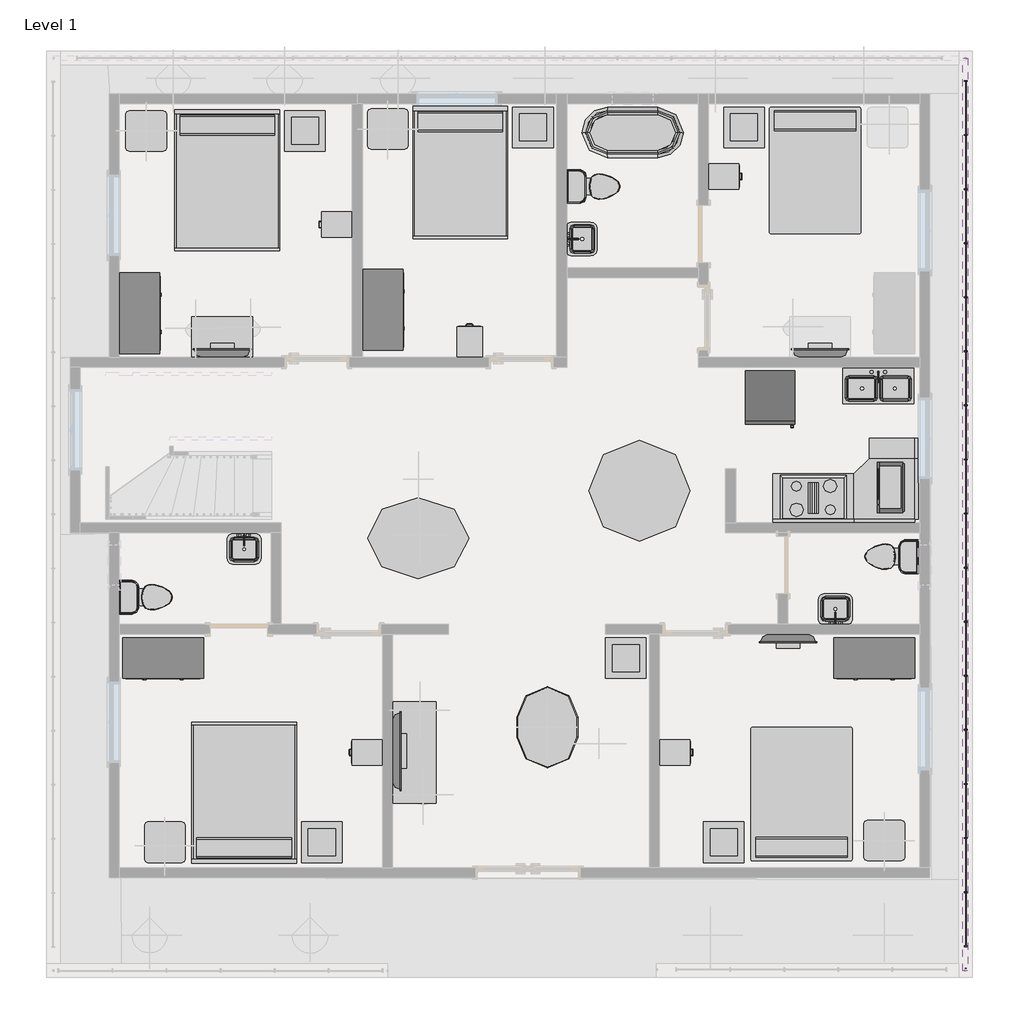
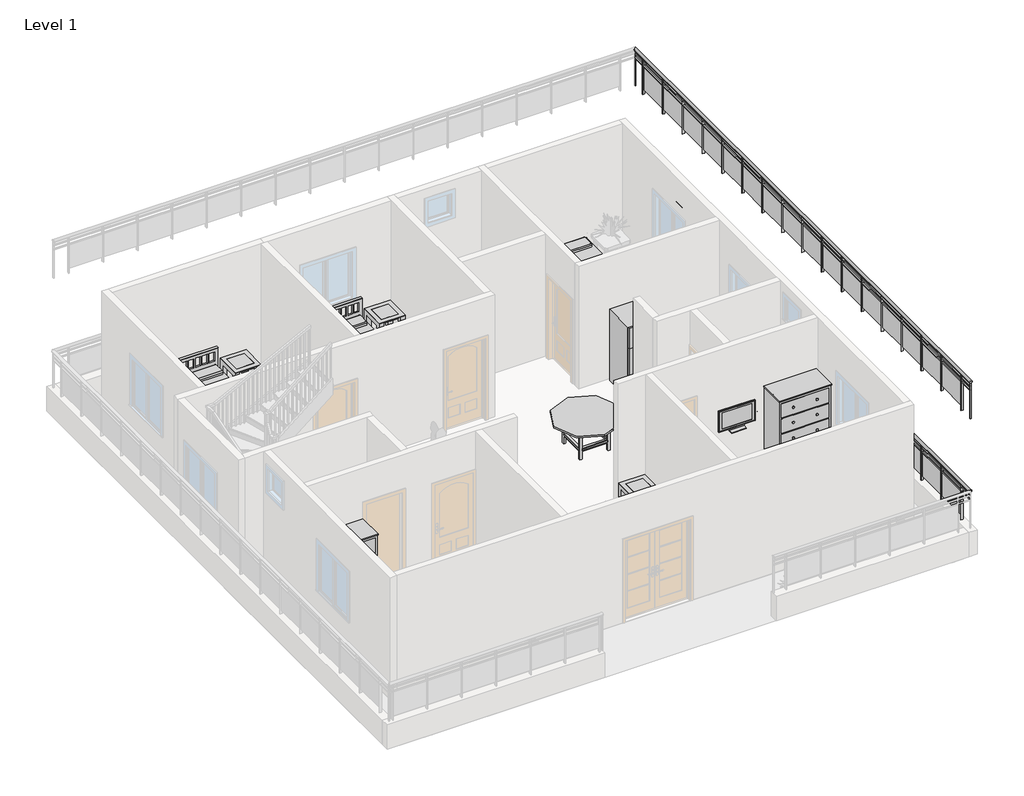
# One storey, part 4 of 5: 34 furniture elements, 11 flow terminals, 3 proxies, 2 railings.
"""IFC4 building model written with IfcOpenShell, lengths in millimetres."""

from ifc_helpers import new_model, si_unit, point, frame, origin, place, context, project, spatial, polyline, ellipse_curve, trimmed, outline, extrude, transform, mapped, element, save
from ifc_brep_helpers import plane_surface, extruded_surface, advanced_brep
from components import proxy_bb1e6e30, proxy_8a8d5ab2, proxy_a13a33b2, flow_terminal_accce45a, flow_terminal_a53be723, flow_terminal_62a433f7, toilet_domestic_3d_toilet_domestic_3d_f7549cf7, toilet_domestic_3d_toilet_domestic_3d_183bbd19, flow_terminal_b374fae2, furniture_096e7f55, furniture_35c09872, furniture_0253826f, furniture_e1791683, furniture_bb55ed6b, furniture_9fa109b2, furniture_56245f3a, furniture_d9bcc661, furniture_b5c51a22, furniture_be1c6672, furniture_bbcc68ce, furniture_cacb7300, furniture_31d08a24, furniture_5341d497, furniture_06ea8467, furniture_3c9f2b99

model = new_model("IFC4")

# Units and contexts
model_context = context("Model", 3, world=origin())
ifc_project = project(units=[si_unit("LENGTHUNIT", "METRE", prefix="MILLI")], contexts=[model_context])

# Site, building, storey
site = spatial("IfcSite", under=ifc_project)
building = spatial("IfcBuilding", under=site)
storey = spatial("IfcBuildingStorey", under=building, Name="Level 1", Elevation=0.0)

# Proxies
placement = place(None, origin())
proxy_shape = proxy_bb1e6e30(model_context)
element("IfcBuildingElementProxy", 1, Name="Cook Top-4 Unit : 36\" x 20\"", ObjectType="Cook Top-4 Unit : 36\" x 20\"", at=placement, inside=storey, context=model_context, shape_type="MappedRepresentation", body=[
    mapped(proxy_shape, transform((-49.0434666, 7731.8216937, 0.0), x_axis=(1.0, 0.0, 0.0), y_axis=(0.0, 1.0, 0.0), z_axis=(0.0, 0.0, 1.0))),
])
proxy_2_shape = proxy_8a8d5ab2(model_context)
element("IfcBuildingElementProxy", 2, Name="Microwave : 30\" x 16\" x 18\"", ObjectType="Microwave : 30\" x 16\" x 18\"", at=placement, inside=storey, context=model_context, shape_type="MappedRepresentation", body=[
    mapped(proxy_2_shape, transform((1472.4370392, 8390.864571, 0.0), x_axis=(0.0, -1.0000000000000002, 0.0), y_axis=(1.0000000000000002, 0.0, 0.0), z_axis=(0.0, 0.0, 1.0))),
])
proxy_3_shape = proxy_a13a33b2(model_context)
element("IfcBuildingElementProxy", 3, Name="Refrigerator : 30\" x 32\" RH", ObjectType="Refrigerator : 30\" x 32\" RH", at=placement, inside=storey, context=model_context, shape_type="MappedRepresentation", body=[
    mapped(proxy_3_shape, transform((-701.8944951, 9254.2341937, 0.0), x_axis=(1.0000000000000007, 0.0, 0.0), y_axis=(0.0, 1.0000000000000007, 0.0), z_axis=(0.0, 0.0, 1.0))),
])

# Flow terminals
flow_terminal_shape = flow_terminal_accce45a(model_context)
element("IfcFlowTerminal", 4, ObjectType="Floor Drain - Round : 5\" Strainer - 2\" Drain", at=placement, inside=storey, context=model_context, shape_type="MappedRepresentation", body=[
    mapped(flow_terminal_shape, transform((-2004.8434666, 12614.9716937, 0.0), x_axis=(1.0, 0.0, 0.0), y_axis=(0.0, 1.0, 0.0), z_axis=(0.0, 0.0, 1.0))),
])
element("IfcFlowTerminal", 5, ObjectType="Floor Drain - Round : 5\" Strainer - 2\" Drain", at=placement, inside=storey, context=model_context, shape_type="MappedRepresentation", body=[
    mapped(flow_terminal_shape, transform((-10259.8434666, 6950.7716937, 0.0), x_axis=(1.0, 0.0, 0.0), y_axis=(0.0, 1.0, 0.0), z_axis=(0.0, 0.0, 1.0))),
])
element("IfcFlowTerminal", 6, ObjectType="Floor Drain - Round : 5\" Strainer - 2\" Drain", at=placement, inside=storey, context=model_context, shape_type="MappedRepresentation", body=[
    mapped(flow_terminal_shape, transform((1322.5565334, 6137.9716937, 0.0), x_axis=(1.0, 0.0, 0.0), y_axis=(0.0, 1.0, 0.0), z_axis=(0.0, 0.0, 1.0))),
])
flow_terminal_2_shape = flow_terminal_a53be723(model_context)
element("IfcFlowTerminal", 7, ObjectType="Sink Kitchen-Double : 42\" x 21\"", at=placement, inside=storey, context=model_context, shape_type="MappedRepresentation", body=[
    mapped(flow_terminal_2_shape, transform((913.1672928, 9412.2262926, 0.0), x_axis=(1.0000000000000004, 0.0, 0.0), y_axis=(0.0, 1.0000000000000004, 0.0), z_axis=(0.0, 0.0, 1.0))),
])
flow_terminal_3_shape = flow_terminal_62a433f7(model_context)
element("IfcFlowTerminal", 8, ObjectType="Sink Vanity-Square : 20\" x 18\"", at=placement, inside=storey, context=model_context, shape_type="MappedRepresentation", body=[
    mapped(flow_terminal_3_shape, transform((-3577.2980655, 11608.6824531, 0.0), x_axis=(0.0, 1.0000000000000002, 0.0), y_axis=(-1.0000000000000002, 0.0, 0.0), z_axis=(0.0, 0.0, 1.0))),
])
element("IfcFlowTerminal", 9, ObjectType="Sink Vanity-Square : 20\" x 18\"", at=placement, inside=storey, context=model_context, shape_type="MappedRepresentation", body=[
    mapped(flow_terminal_3_shape, transform((-8624.5327072, 7011.9262926, 0.0), x_axis=(1.0, 0.0, 0.0), y_axis=(0.0, 1.0, 0.0), z_axis=(0.0, 0.0, 1.0))),
])
element("IfcFlowTerminal", 10, ObjectType="Sink Vanity-Square : 20\" x 18\"", at=placement, inside=storey, context=model_context, shape_type="MappedRepresentation", body=[
    mapped(flow_terminal_3_shape, transform((296.845774, 6013.3170948, 0.0), x_axis=(-1.0, 0.0, 0.0), y_axis=(0.0, -1.0, 0.0), z_axis=(0.0, 0.0, 1.0))),
])
toilet_domestic_3d_toilet_domestic_3d_shape = toilet_domestic_3d_toilet_domestic_3d_f7549cf7(model_context)
toilet_domestic_3d_toilet_domestic_3d_2_shape = toilet_domestic_3d_toilet_domestic_3d_183bbd19(model_context)
element("IfcFlowTerminal", 11, ObjectType="Toilet-Domestic-3D : Toilet-Domestic-3D", at=placement, inside=storey, context=model_context, shape_type="MappedRepresentation", body=[
    mapped(toilet_domestic_3d_toilet_domestic_3d_shape, transform((-3262.7474393, 12411.7716937, 0.0), x_axis=(0.0, 1.0000000000000002, 0.0), y_axis=(-1.0000000000000002, 0.0, 0.0), z_axis=(0.0, 0.0, 1.0))),
    mapped(toilet_domestic_3d_toilet_domestic_3d_2_shape, transform((-3262.7474393, 12411.7716937, 0.0), x_axis=(0.0, 1.0000000000000002, 0.0), y_axis=(-1.0000000000000002, 0.0, 0.0), z_axis=(0.0, 0.0, 1.0))),
])
element("IfcFlowTerminal", 12, ObjectType="Toilet-Domestic-3D : Toilet-Domestic-3D", at=placement, inside=storey, context=model_context, shape_type="MappedRepresentation", body=[
    mapped(toilet_domestic_3d_toilet_domestic_3d_shape, transform((-9993.7474393, 6239.5716937, 0.0), x_axis=(0.0, 1.0000000000000002, 0.0), y_axis=(-1.0000000000000002, 0.0, 0.0), z_axis=(0.0, 0.0, 1.0))),
    mapped(toilet_domestic_3d_toilet_domestic_3d_2_shape, transform((-9993.7474393, 6239.5716937, 0.0), x_axis=(0.0, 1.0000000000000002, 0.0), y_axis=(-1.0000000000000002, 0.0, 0.0), z_axis=(0.0, 0.0, 1.0))),
])
element("IfcFlowTerminal", 13, ObjectType="Toilet-Domestic-3D : Toilet-Domestic-3D", at=placement, inside=storey, context=model_context, shape_type="MappedRepresentation", body=[
    mapped(toilet_domestic_3d_toilet_domestic_3d_shape, transform((1031.060506, 6849.1716937, 0.0), x_axis=(0.0, -1.0000000000000002, 0.0), y_axis=(1.0000000000000002, 0.0, 0.0), z_axis=(0.0, 0.0, 1.0))),
    mapped(toilet_domestic_3d_toilet_domestic_3d_2_shape, transform((1031.060506, 6849.1716937, 0.0), x_axis=(0.0, -1.0000000000000002, 0.0), y_axis=(1.0000000000000002, 0.0, 0.0), z_axis=(0.0, 0.0, 1.0))),
])
flow_terminal_4_shape = flow_terminal_b374fae2(model_context)
element("IfcFlowTerminal", 14, ObjectType="Tub-Free Standing-3D : 30\" x 60\"", at=placement, inside=storey, context=model_context, shape_type="MappedRepresentation", body=[
    mapped(flow_terminal_4_shape, transform((-2766.8434666, 13224.5716937, 0.0), x_axis=(0.0, 1.0000000000000002, 0.0), y_axis=(-1.0000000000000002, 0.0, 0.0), z_axis=(0.0, 0.0, 1.0))),
])

# Furniture
furniture_shape = furniture_096e7f55(model_context)
element("IfcFurniture", 15, ObjectType="Bed-Shaker : Double 56\" x 78\"", at=placement, inside=storey, context=model_context, shape_type="MappedRepresentation", body=[
    mapped(furniture_shape, transform((-5338.5934666, 13605.5716937, 0.0), x_axis=(1.0, 0.0, 0.0), y_axis=(0.0, 1.0, 0.0), z_axis=(0.0, 0.0, 1.0))),
])
furniture_2_shape = furniture_35c09872(model_context)
element("IfcFurniture", 16, ObjectType="Bed-Shaker : Queen 62\" x 83\"", at=placement, inside=storey, context=model_context, shape_type="MappedRepresentation", body=[
    mapped(furniture_2_shape, transform((-8843.7934666, 13554.7716937, 0.0), x_axis=(1.0, 0.0, 0.0), y_axis=(0.0, 1.0, 0.0), z_axis=(0.0, 0.0, 1.0))),
])
element("IfcFurniture", 17, ObjectType="Bed-Shaker : Queen 62\" x 83\"", at=placement, inside=storey, context=model_context, shape_type="MappedRepresentation", body=[
    mapped(furniture_2_shape, transform((-8627.8934666, 2251.7716937, 0.0), x_axis=(-1.0000000000000002, 0.0, 0.0), y_axis=(0.0, -1.0000000000000002, 0.0), z_axis=(0.0, 0.0, 1.0))),
])
furniture_3_shape = furniture_0253826f(model_context)
element("IfcFurniture", 18, ObjectType="Bed-Standard : Double 54\" x 75\"", at=placement, inside=storey, context=model_context, shape_type="MappedRepresentation", body=[
    mapped(furniture_3_shape, transform((-295.1319912, 12698.6667757, 0.0), x_axis=(1.0, 0.0, 0.0), y_axis=(0.0, 1.0, 0.0), z_axis=(0.0, 0.0, 1.0))),
])
furniture_4_shape = furniture_e1791683(model_context)
element("IfcFurniture", 19, ObjectType="Bed-Standard : Queen 60\" x 79\"", at=placement, inside=storey, context=model_context, shape_type="MappedRepresentation", body=[
    mapped(furniture_4_shape, transform((44.645058, 3234.8766117, 0.0), x_axis=(-1.0, 0.0, 0.0), y_axis=(0.0, -1.0, 0.0), z_axis=(0.0, 0.0, 1.0))),
])
furniture_5_shape = furniture_bb55ed6b(model_context)
element("IfcFurniture", 20, ObjectType="Cabinet-File 2 Drawer : 15\" x 18\"", at=placement, inside=storey, context=model_context, shape_type="MappedRepresentation", body=[
    mapped(furniture_5_shape, transform((-7069.7091665, 11712.3752467, 0.0), x_axis=(0.0, -1.0000000000000004, 0.0), y_axis=(1.0000000000000004, 0.0, 0.0), z_axis=(0.0, 0.0, 1.0))),
])
element("IfcFurniture", 21, ObjectType="Cabinet-File 2 Drawer : 15\" x 18\"", at=placement, inside=storey, context=model_context, shape_type="MappedRepresentation", body=[
    mapped(furniture_5_shape, transform((-5345.8399136, 9932.8373936, 0.0), x_axis=(-1.0, 0.0, 0.0), y_axis=(0.0, -1.0, 0.0), z_axis=(0.0, 0.0, 1.0))),
])
element("IfcFurniture", 22, ObjectType="Cabinet-File 2 Drawer : 15\" x 18\"", at=placement, inside=storey, context=model_context, shape_type="MappedRepresentation", body=[
    mapped(furniture_5_shape, transform((-1537.3777667, 12692.0681407, 0.0), x_axis=(0.0, 1.0000000000000002, 0.0), y_axis=(-1.0000000000000002, 0.0, 0.0), z_axis=(0.0, 0.0, 1.0))),
])
element("IfcFurniture", 23, ObjectType="Cabinet-File 2 Drawer : 15\" x 18\"", at=placement, inside=storey, context=model_context, shape_type="MappedRepresentation", body=[
    mapped(furniture_5_shape, transform((-6612.5091665, 3778.8994064, 0.0), x_axis=(0.0, -1.0, 0.0), y_axis=(1.0, 0.0, 0.0), z_axis=(0.0, 0.0, 1.0))),
])
element("IfcFurniture", 24, ObjectType="Cabinet-File 2 Drawer : 15\" x 18\"", at=placement, inside=storey, context=model_context, shape_type="MappedRepresentation", body=[
    mapped(furniture_5_shape, transform((-2273.9777667, 4034.6923005, 0.0), x_axis=(0.0, 1.0000000000000009, 0.0), y_axis=(-1.0000000000000009, 0.0, 0.0), z_axis=(0.0, 0.0, 1.0))),
])
furniture_6_shape = furniture_9fa109b2(model_context)
element("IfcFurniture", 25, ObjectType="Dresser : 48\" x 72\" x 24\"", at=placement, inside=storey, context=model_context, shape_type="MappedRepresentation", body=[
    mapped(furniture_6_shape, transform((-10546.8064207, 10775.9649535, 0.0), x_axis=(0.0, 1.0, 0.0), y_axis=(-1.0, 0.0, 0.0), z_axis=(0.0, 0.0, 1.0))),
])
element("IfcFurniture", 26, ObjectType="Dresser : 48\" x 72\" x 24\"", at=placement, inside=storey, context=model_context, shape_type="MappedRepresentation", body=[
    mapped(furniture_6_shape, transform((-6889.2064207, 10826.7649535, 0.0), x_axis=(0.0, 1.0, 0.0), y_axis=(-1.0, 0.0, 0.0), z_axis=(0.0, 0.0, 1.0))),
])
element("IfcFurniture", 27, ObjectType="Dresser : 48\" x 72\" x 24\"", at=placement, inside=storey, context=model_context, shape_type="MappedRepresentation", body=[
    mapped(furniture_6_shape, transform((-9558.8502068, 5688.3346478, 0.0), x_axis=(1.0, 0.0, 0.0), y_axis=(0.0, 1.0, 0.0), z_axis=(0.0, 0.0, 1.0))),
])
element("IfcFurniture", 28, ObjectType="Dresser : 48\" x 72\" x 24\"", at=placement, inside=storey, context=model_context, shape_type="MappedRepresentation", body=[
    mapped(furniture_6_shape, transform((1134.5497932, 5688.3346478, 0.0), x_axis=(1.0, 0.0, 0.0), y_axis=(0.0, 1.0, 0.0), z_axis=(0.0, 0.0, 1.0))),
])
furniture_7_shape = furniture_56245f3a(model_context)
element("IfcFurniture", 29, ObjectType="TV - Flat Screen : 32\"", at=placement, inside=storey, context=model_context, shape_type="MappedRepresentation", body=[
    mapped(furniture_7_shape, transform((-8942.9879808, 9904.9103174, 1041.4), x_axis=(-1.0000000000000004, 0.0, 0.0), y_axis=(0.0, -1.0000000000000004, 0.0), z_axis=(0.0, 0.0, 1.0))),
])
element("IfcFurniture", 30, ObjectType="TV - Flat Screen : 32\"", at=placement, inside=storey, context=model_context, shape_type="MappedRepresentation", body=[
    mapped(furniture_7_shape, transform((48.6120192, 9904.9103174, 1041.4), x_axis=(-1.0000000000000004, 0.0, 0.0), y_axis=(0.0, -1.0000000000000004, 0.0), z_axis=(0.0, 0.0, 1.0))),
])
element("IfcFurniture", 31, ObjectType="TV - Flat Screen : 32\"", at=placement, inside=storey, context=model_context, shape_type="MappedRepresentation", body=[
    mapped(furniture_7_shape, transform((-426.0989525, 5622.2330701, 1041.4), x_axis=(1.0, 0.0, 0.0), y_axis=(0.0, 1.0, 0.0), z_axis=(0.0, 0.0, 1.0))),
])
furniture_8_shape = furniture_d9bcc661(model_context)
element("IfcFurniture", 32, ObjectType="TV - Flat Screen : 46\"", at=placement, inside=storey, context=model_context, shape_type="MappedRepresentation", body=[
    mapped(furniture_8_shape, transform((-6315.104843, 3932.1162078, 1041.4), x_axis=(0.0, 1.0000000000000002, 0.0), y_axis=(-1.0000000000000002, 0.0, 0.0), z_axis=(0.0, 0.0, 1.0))),
])
furniture_9_shape = furniture_b5c51a22(model_context)
element("IfcFurniture", 33, ObjectType="Table-Coffee : 24\" x 24\" x 24\"", at=placement, inside=storey, context=model_context, shape_type="MappedRepresentation", body=[
    mapped(furniture_9_shape, transform((-7712.7092333, 13154.7606159, 0.0), x_axis=(1.0, 0.0, 0.0), y_axis=(0.0, 1.0, 0.0), z_axis=(0.0, 0.0, 1.0))),
])
element("IfcFurniture", 34, ObjectType="Table-Coffee : 24\" x 24\" x 24\"", at=placement, inside=storey, context=model_context, shape_type="MappedRepresentation", body=[
    mapped(furniture_9_shape, transform((-4283.7092333, 13205.5606159, 0.0), x_axis=(1.0, 0.0, 0.0), y_axis=(0.0, 1.0, 0.0), z_axis=(0.0, 0.0, 1.0))),
])
element("IfcFurniture", 35, ObjectType="Table-Coffee : 24\" x 24\" x 24\"", at=placement, inside=storey, context=model_context, shape_type="MappedRepresentation", body=[
    mapped(furniture_9_shape, transform((-1108.7092333, 13205.5606159, 0.0), x_axis=(1.0, 0.0, 0.0), y_axis=(0.0, 1.0, 0.0), z_axis=(0.0, 0.0, 1.0))),
])
element("IfcFurniture", 36, ObjectType="Table-Coffee : 24\" x 24\" x 24\"", at=placement, inside=storey, context=model_context, shape_type="MappedRepresentation", body=[
    mapped(furniture_9_shape, transform((-7458.7092333, 2461.3606159, 0.0), x_axis=(1.0, 0.0, 0.0), y_axis=(0.0, 1.0, 0.0), z_axis=(0.0, 0.0, 1.0))),
])
element("IfcFurniture", 37, ObjectType="Table-Coffee : 24\" x 24\" x 24\"", at=placement, inside=storey, context=model_context, shape_type="MappedRepresentation", body=[
    mapped(furniture_9_shape, transform((-1413.5092333, 2461.3606159, 0.0), x_axis=(1.0, 0.0, 0.0), y_axis=(0.0, 1.0, 0.0), z_axis=(0.0, 0.0, 1.0))),
])
element("IfcFurniture", 38, ObjectType="Table-Coffee : 24\" x 24\" x 24\"", at=placement, inside=storey, context=model_context, shape_type="MappedRepresentation", body=[
    mapped(furniture_9_shape, transform((-2886.7092333, 5229.9606159, 0.0), x_axis=(1.0, 0.0, 0.0), y_axis=(0.0, 1.0, 0.0), z_axis=(0.0, 0.0, 1.0))),
])
furniture_10_shape = furniture_be1c6672(model_context)
element("IfcFurniture", 39, ObjectType="Table-Dining Oval : 36\" x 48\"", at=placement, inside=storey, context=model_context, shape_type="MappedRepresentation", body=[
    mapped(furniture_10_shape, transform((-4407.6418273, 4685.5913658, 0.0), x_axis=(0.0, 1.0000000000000002, 0.0), y_axis=(-1.0000000000000002, 0.0, 0.0), z_axis=(0.0, 0.0, 1.0))),
])
furniture_11_shape = furniture_bbcc68ce(model_context)
element("IfcFurniture", 40, ObjectType="Table-Dining Round w Chairs : 60\" Diameter", at=placement, inside=storey, context=model_context, shape_type="MappedRepresentation", body=[
    mapped(furniture_11_shape, transform((-2768.9254338, 8024.6503822, 0.0), x_axis=(1.0, 0.0, 0.0), y_axis=(0.0, 1.0, 0.0), z_axis=(0.0, 0.0, 1.0))),
])
furniture_12_shape = furniture_cacb7300(model_context)
element("IfcFurniture", 41, ObjectType="Table-Ellipse : 60\" x 48\"", at=placement, inside=storey, context=model_context, shape_type="MappedRepresentation", body=[
    mapped(furniture_12_shape, transform((-5992.6434666, 7128.5716937, 0.0), x_axis=(1.0, 0.0, 0.0), y_axis=(0.0, 1.0, 0.0), z_axis=(0.0, 0.0, 1.0))),
])
furniture_13_shape = furniture_31d08a24(model_context)
element("IfcFurniture", 42, ObjectType="Table-End : 24\" x 24\"", at=placement, inside=storey, context=model_context, shape_type="MappedRepresentation", body=[
    mapped(furniture_13_shape, transform((-10390.5770969, 13097.5716937, 0.0), x_axis=(1.0, 0.0, 0.0), y_axis=(0.0, 1.0, 0.0), z_axis=(0.0, 0.0, 1.0))),
])
element("IfcFurniture", 43, ObjectType="Table-End : 24\" x 24\"", at=placement, inside=storey, context=model_context, shape_type="MappedRepresentation", body=[
    mapped(furniture_13_shape, transform((-6758.3770969, 13122.9716937, 0.0), x_axis=(1.0, 0.0, 0.0), y_axis=(0.0, 1.0, 0.0), z_axis=(0.0, 0.0, 1.0))),
])
element("IfcFurniture", 44, ObjectType="Table-End : 24\" x 24\"", at=placement, inside=storey, context=model_context, shape_type="MappedRepresentation", body=[
    mapped(furniture_13_shape, transform((-10111.1770969, 2404.1716937, 0.0), x_axis=(1.0, 0.0, 0.0), y_axis=(0.0, 1.0, 0.0), z_axis=(0.0, 0.0, 1.0))),
])
element("IfcFurniture", 45, ObjectType="Table-End : 24\" x 24\"", at=placement, inside=storey, context=model_context, shape_type="MappedRepresentation", body=[
    mapped(furniture_13_shape, transform((709.2229031, 2429.5716937, 0.0), x_axis=(1.0, 0.0, 0.0), y_axis=(0.0, 1.0, 0.0), z_axis=(0.0, 0.0, 1.0))),
])
furniture_14_shape = furniture_5341d497(model_context)
element("IfcFurniture", 46, ObjectType="Table-Rectangular : 72\" x 30\"", at=placement, inside=storey, context=model_context, shape_type="MappedRepresentation", body=[
    mapped(furniture_14_shape, transform((-8939.0434666, 10151.1716937, 0.0), x_axis=(1.0, 0.0, 0.0), y_axis=(0.0, 1.0, 0.0), z_axis=(0.0, 0.0, 1.0))),
])
furniture_15_shape = furniture_06ea8467(model_context)
element("IfcFurniture", 47, ObjectType="Table-Rectangular : 72\" x 30\" 2", at=placement, inside=storey, context=model_context, shape_type="MappedRepresentation", body=[
    mapped(furniture_15_shape, transform((-6068.8434666, 3906.7958535, 0.0), x_axis=(0.0, 1.0000000000000002, 0.0), y_axis=(-1.0000000000000002, 0.0, 0.0), z_axis=(0.0, 0.0, 1.0))),
])
furniture_16_shape = furniture_3c9f2b99(model_context)
element("IfcFurniture", 48, ObjectType="Work Station Cubicle : 96\" x 96\"", at=placement, inside=storey, context=model_context, shape_type="MappedRepresentation", body=[
    mapped(furniture_16_shape, transform((1394.0247812, 6862.1486861, 0.0), x_axis=(-1.0000000000000004, 0.0, 0.0), y_axis=(0.0, -1.0000000000000004, 0.0), z_axis=(0.0, 0.0, 1.0))),
])

# Railings
element("IfcRailing", 49, ObjectType="Glass Panel - Bottom Fill", at=placement, inside=storey, context=model_context, shape_type="SolidModel", body=[
    advanced_brep(
    [(2275.0565334, 14342.1716937, 4267.2), (2198.8565334, 14342.1716937, 4267.2), (2275.0565334, 626.1716937, 4267.2), (2198.8565334, 626.1716937, 4267.2)],
    [
        (0, 1, ellipse_curve(frame((2236.9565334, 14342.1716937, 4267.2), z_axis=(0.0, 1.0, 0.0), x_axis=(-1.0, 0.0, 0.0)), 38.1, 28.575)),
        (1, 0, ellipse_curve(frame((2236.9565334, 14342.1716937, 4267.2), z_axis=(0.0, 1.0, 0.0), x_axis=(-1.0, 0.0, 0.0)), 38.1, 28.575)),
        (2, 3, ellipse_curve(frame((2236.9565334, 626.1716937, 4267.2), z_axis=(0.0, -1.0, 0.0), x_axis=(-1.0, 0.0, 0.0)), 38.1, 28.575)),
        (3, 2, ellipse_curve(frame((2236.9565334, 626.1716937, 4267.2), z_axis=(0.0, -1.0, 0.0), x_axis=(-1.0, 0.0, 0.0)), 38.1, 28.575)),
        (0, 2),
        (3, 1),
    ],
    [
        plane_surface(frame((2236.9565334, 14342.1716937, 4267.2), z_axis=(0.0, 1.0, 0.0), x_axis=(0.0, 0.0, -1.0))),
        plane_surface(frame((2236.9565334, 626.1716937, 4267.2), z_axis=(0.0, -1.0, 0.0), x_axis=(0.0, 0.0, -1.0))),
        extruded_surface(trimmed(ellipse_curve(frame((2236.9565334, 626.1716937, 4267.2), z_axis=(0.0, 1.0, 0.0), x_axis=(-1.0, 0.0, 0.0)), 38.1, 28.575), [point((2275.0565334, 626.1716937, 4267.2))], [point((2198.8565334, 626.1716937, 4267.2))], True, "CARTESIAN"), (0.0, 13716.0, 0.0), 13716.0),
        extruded_surface(trimmed(ellipse_curve(frame((2236.9565334, 626.1716937, 4267.2), z_axis=(0.0, 1.0, 0.0), x_axis=(-1.0, 0.0, 0.0)), 38.1, 28.575), [point((2198.8565334, 626.1716937, 4267.2))], [point((2275.0565334, 626.1716937, 4267.2))], True, "CARTESIAN"), (0.0, 13716.0, 0.0), 13716.0),
    ],
    [
        (0, [[1, 2]]),
        (1, [[3, 4]]),
        (2, [[-1, 5, -4, 6]]),
        (3, [[-2, -6, -3, -5]]),
    ],
),
    extrude(outline(polyline([(2224.2565334, 14342.1716937), (2249.6565334, 14342.1716937), (2249.6565334, 626.1716937), (2224.2565334, 626.1716937), (2224.2565334, 14342.1716937)])), frame((0.0, 0.0, 4152.9), z_axis=(0.0, 0.0, 1.0), x_axis=(1.0, 0.0, 0.0)), (0.0, 0.0, 1.0), 25.4),
    extrude(outline(polyline([(2224.2565334, 14342.1716937), (2249.6565334, 14342.1716937), (2249.6565334, 626.1716937), (2224.2565334, 626.1716937), (2224.2565334, 14342.1716937)])), frame((0.0, 0.0, 4051.3), z_axis=(0.0, 0.0, 1.0), x_axis=(1.0, 0.0, 0.0)), (0.0, 0.0, 1.0), 25.4),
    extrude(outline(polyline([(2211.5565334, 988.1216937), (2262.3565334, 988.1216937), (2262.3565334, 975.4216937), (2211.5565334, 975.4216937), (2211.5565334, 988.1216937)])), frame((0.0, 0.0, 3352.8), z_axis=(0.0, 0.0, 1.0), x_axis=(1.0, 0.0, 0.0)), (0.0, 0.0, 1.0), 885.6788223),
    extrude(outline(polyline([(2243.4916904, 1794.5716937), (2243.4916904, 981.7716937), (2237.1416904, 981.7716937), (2237.1416904, 1794.5716937), (2243.4916904, 1794.5716937)])), frame((0.0, 0.0, 3454.4), z_axis=(0.0, 0.0, 1.0), x_axis=(1.0, 0.0, 0.0)), (0.0, 0.0, 1.0), 596.9),
    extrude(outline(polyline([(2211.5565334, 1800.9216937), (2262.3565334, 1800.9216937), (2262.3565334, 1788.2216937), (2211.5565334, 1788.2216937), (2211.5565334, 1800.9216937)])), frame((0.0, 0.0, 3352.8), z_axis=(0.0, 0.0, 1.0), x_axis=(1.0, 0.0, 0.0)), (0.0, 0.0, 1.0), 885.6788223),
    extrude(outline(polyline([(2243.4916904, 2607.3716937), (2243.4916904, 1794.5716937), (2237.1416904, 1794.5716937), (2237.1416904, 2607.3716937), (2243.4916904, 2607.3716937)])), frame((0.0, 0.0, 3454.4), z_axis=(0.0, 0.0, 1.0), x_axis=(1.0, 0.0, 0.0)), (0.0, 0.0, 1.0), 596.9),
    extrude(outline(polyline([(2211.5565334, 2613.7216937), (2262.3565334, 2613.7216937), (2262.3565334, 2601.0216937), (2211.5565334, 2601.0216937), (2211.5565334, 2613.7216937)])), frame((0.0, 0.0, 3352.8), z_axis=(0.0, 0.0, 1.0), x_axis=(1.0, 0.0, 0.0)), (0.0, 0.0, 1.0), 885.6788223),
    extrude(outline(polyline([(2243.4916904, 3420.1716937), (2243.4916904, 2607.3716937), (2237.1416904, 2607.3716937), (2237.1416904, 3420.1716937), (2243.4916904, 3420.1716937)])), frame((0.0, 0.0, 3454.4), z_axis=(0.0, 0.0, 1.0), x_axis=(1.0, 0.0, 0.0)), (0.0, 0.0, 1.0), 596.9),
    extrude(outline(polyline([(2211.5565334, 3426.5216937), (2262.3565334, 3426.5216937), (2262.3565334, 3413.8216937), (2211.5565334, 3413.8216937), (2211.5565334, 3426.5216937)])), frame((0.0, 0.0, 3352.8), z_axis=(0.0, 0.0, 1.0), x_axis=(1.0, 0.0, 0.0)), (0.0, 0.0, 1.0), 885.6788223),
    extrude(outline(polyline([(2243.4916904, 4232.9716937), (2243.4916904, 3420.1716937), (2237.1416904, 3420.1716937), (2237.1416904, 4232.9716937), (2243.4916904, 4232.9716937)])), frame((0.0, 0.0, 3454.4), z_axis=(0.0, 0.0, 1.0), x_axis=(1.0, 0.0, 0.0)), (0.0, 0.0, 1.0), 596.9),
    extrude(outline(polyline([(2211.5565334, 4239.3216937), (2262.3565334, 4239.3216937), (2262.3565334, 4226.6216937), (2211.5565334, 4226.6216937), (2211.5565334, 4239.3216937)])), frame((0.0, 0.0, 3352.8), z_axis=(0.0, 0.0, 1.0), x_axis=(1.0, 0.0, 0.0)), (0.0, 0.0, 1.0), 885.6788223),
    extrude(outline(polyline([(2243.4916904, 5045.7716937), (2243.4916904, 4232.9716937), (2237.1416904, 4232.9716937), (2237.1416904, 5045.7716937), (2243.4916904, 5045.7716937)])), frame((0.0, 0.0, 3454.4), z_axis=(0.0, 0.0, 1.0), x_axis=(1.0, 0.0, 0.0)), (0.0, 0.0, 1.0), 596.9),
    extrude(outline(polyline([(2211.5565334, 5052.1216937), (2262.3565334, 5052.1216937), (2262.3565334, 5039.4216937), (2211.5565334, 5039.4216937), (2211.5565334, 5052.1216937)])), frame((0.0, 0.0, 3352.8), z_axis=(0.0, 0.0, 1.0), x_axis=(1.0, 0.0, 0.0)), (0.0, 0.0, 1.0), 885.6788223),
    extrude(outline(polyline([(2243.4916904, 5858.5716937), (2243.4916904, 5045.7716937), (2237.1416904, 5045.7716937), (2237.1416904, 5858.5716937), (2243.4916904, 5858.5716937)])), frame((0.0, 0.0, 3454.4), z_axis=(0.0, 0.0, 1.0), x_axis=(1.0, 0.0, 0.0)), (0.0, 0.0, 1.0), 596.9),
    extrude(outline(polyline([(2211.5565334, 5864.9216937), (2262.3565334, 5864.9216937), (2262.3565334, 5852.2216937), (2211.5565334, 5852.2216937), (2211.5565334, 5864.9216937)])), frame((0.0, 0.0, 3352.8), z_axis=(0.0, 0.0, 1.0), x_axis=(1.0, 0.0, 0.0)), (0.0, 0.0, 1.0), 885.6788223),
    extrude(outline(polyline([(2243.4916904, 6671.3716937), (2243.4916904, 5858.5716937), (2237.1416904, 5858.5716937), (2237.1416904, 6671.3716937), (2243.4916904, 6671.3716937)])), frame((0.0, 0.0, 3454.4), z_axis=(0.0, 0.0, 1.0), x_axis=(1.0, 0.0, 0.0)), (0.0, 0.0, 1.0), 596.9),
    extrude(outline(polyline([(2211.5565334, 6677.7216937), (2262.3565334, 6677.7216937), (2262.3565334, 6665.0216937), (2211.5565334, 6665.0216937), (2211.5565334, 6677.7216937)])), frame((0.0, 0.0, 3352.8), z_axis=(0.0, 0.0, 1.0), x_axis=(1.0, 0.0, 0.0)), (0.0, 0.0, 1.0), 885.6788223),
    extrude(outline(polyline([(2243.4916904, 7484.1716937), (2243.4916904, 6671.3716937), (2237.1416904, 6671.3716937), (2237.1416904, 7484.1716937), (2243.4916904, 7484.1716937)])), frame((0.0, 0.0, 3454.4), z_axis=(0.0, 0.0, 1.0), x_axis=(1.0, 0.0, 0.0)), (0.0, 0.0, 1.0), 596.9),
    extrude(outline(polyline([(2211.5565334, 7490.5216937), (2262.3565334, 7490.5216937), (2262.3565334, 7477.8216937), (2211.5565334, 7477.8216937), (2211.5565334, 7490.5216937)])), frame((0.0, 0.0, 3352.8), z_axis=(0.0, 0.0, 1.0), x_axis=(1.0, 0.0, 0.0)), (0.0, 0.0, 1.0), 885.6788223),
    extrude(outline(polyline([(2243.4916904, 8296.9716937), (2243.4916904, 7484.1716937), (2237.1416904, 7484.1716937), (2237.1416904, 8296.9716937), (2243.4916904, 8296.9716937)])), frame((0.0, 0.0, 3454.4), z_axis=(0.0, 0.0, 1.0), x_axis=(1.0, 0.0, 0.0)), (0.0, 0.0, 1.0), 596.9),
    extrude(outline(polyline([(2211.5565334, 8303.3216937), (2262.3565334, 8303.3216937), (2262.3565334, 8290.6216937), (2211.5565334, 8290.6216937), (2211.5565334, 8303.3216937)])), frame((0.0, 0.0, 3352.8), z_axis=(0.0, 0.0, 1.0), x_axis=(1.0, 0.0, 0.0)), (0.0, 0.0, 1.0), 885.6788223),
    extrude(outline(polyline([(2243.4916904, 9109.7716937), (2243.4916904, 8296.9716937), (2237.1416904, 8296.9716937), (2237.1416904, 9109.7716937), (2243.4916904, 9109.7716937)])), frame((0.0, 0.0, 3454.4), z_axis=(0.0, 0.0, 1.0), x_axis=(1.0, 0.0, 0.0)), (0.0, 0.0, 1.0), 596.9),
    extrude(outline(polyline([(2211.5565334, 9116.1216937), (2262.3565334, 9116.1216937), (2262.3565334, 9103.4216937), (2211.5565334, 9103.4216937), (2211.5565334, 9116.1216937)])), frame((0.0, 0.0, 3352.8), z_axis=(0.0, 0.0, 1.0), x_axis=(1.0, 0.0, 0.0)), (0.0, 0.0, 1.0), 885.6788223),
    extrude(outline(polyline([(2243.4916904, 9922.5716937), (2243.4916904, 9109.7716937), (2237.1416904, 9109.7716937), (2237.1416904, 9922.5716937), (2243.4916904, 9922.5716937)])), frame((0.0, 0.0, 3454.4), z_axis=(0.0, 0.0, 1.0), x_axis=(1.0, 0.0, 0.0)), (0.0, 0.0, 1.0), 596.9),
    extrude(outline(polyline([(2211.5565334, 9928.9216937), (2262.3565334, 9928.9216937), (2262.3565334, 9916.2216937), (2211.5565334, 9916.2216937), (2211.5565334, 9928.9216937)])), frame((0.0, 0.0, 3352.8), z_axis=(0.0, 0.0, 1.0), x_axis=(1.0, 0.0, 0.0)), (0.0, 0.0, 1.0), 885.6788223),
    extrude(outline(polyline([(2243.4916904, 10735.3716937), (2243.4916904, 9922.5716937), (2237.1416904, 9922.5716937), (2237.1416904, 10735.3716937), (2243.4916904, 10735.3716937)])), frame((0.0, 0.0, 3454.4), z_axis=(0.0, 0.0, 1.0), x_axis=(1.0, 0.0, 0.0)), (0.0, 0.0, 1.0), 596.9),
    extrude(outline(polyline([(2211.5565334, 10741.7216937), (2262.3565334, 10741.7216937), (2262.3565334, 10729.0216937), (2211.5565334, 10729.0216937), (2211.5565334, 10741.7216937)])), frame((0.0, 0.0, 3352.8), z_axis=(0.0, 0.0, 1.0), x_axis=(1.0, 0.0, 0.0)), (0.0, 0.0, 1.0), 885.6788223),
    extrude(outline(polyline([(2243.4916904, 11548.1716937), (2243.4916904, 10735.3716937), (2237.1416904, 10735.3716937), (2237.1416904, 11548.1716937), (2243.4916904, 11548.1716937)])), frame((0.0, 0.0, 3454.4), z_axis=(0.0, 0.0, 1.0), x_axis=(1.0, 0.0, 0.0)), (0.0, 0.0, 1.0), 596.9),
    extrude(outline(polyline([(2211.5565334, 11554.5216937), (2262.3565334, 11554.5216937), (2262.3565334, 11541.8216937), (2211.5565334, 11541.8216937), (2211.5565334, 11554.5216937)])), frame((0.0, 0.0, 3352.8), z_axis=(0.0, 0.0, 1.0), x_axis=(1.0, 0.0, 0.0)), (0.0, 0.0, 1.0), 885.6788223),
    extrude(outline(polyline([(2243.4916904, 12360.9716937), (2243.4916904, 11548.1716937), (2237.1416904, 11548.1716937), (2237.1416904, 12360.9716937), (2243.4916904, 12360.9716937)])), frame((0.0, 0.0, 3454.4), z_axis=(0.0, 0.0, 1.0), x_axis=(1.0, 0.0, 0.0)), (0.0, 0.0, 1.0), 596.9),
    extrude(outline(polyline([(2211.5565334, 12367.3216937), (2262.3565334, 12367.3216937), (2262.3565334, 12354.6216937), (2211.5565334, 12354.6216937), (2211.5565334, 12367.3216937)])), frame((0.0, 0.0, 3352.8), z_axis=(0.0, 0.0, 1.0), x_axis=(1.0, 0.0, 0.0)), (0.0, 0.0, 1.0), 885.6788223),
    extrude(outline(polyline([(2243.4916904, 13173.7716937), (2243.4916904, 12360.9716937), (2237.1416904, 12360.9716937), (2237.1416904, 13173.7716937), (2243.4916904, 13173.7716937)])), frame((0.0, 0.0, 3454.4), z_axis=(0.0, 0.0, 1.0), x_axis=(1.0, 0.0, 0.0)), (0.0, 0.0, 1.0), 596.9),
    extrude(outline(polyline([(2211.5565334, 13180.1216937), (2262.3565334, 13180.1216937), (2262.3565334, 13167.4216937), (2211.5565334, 13167.4216937), (2211.5565334, 13180.1216937)])), frame((0.0, 0.0, 3352.8), z_axis=(0.0, 0.0, 1.0), x_axis=(1.0, 0.0, 0.0)), (0.0, 0.0, 1.0), 885.6788223),
    extrude(outline(polyline([(2243.4916904, 13986.5716937), (2243.4916904, 13173.7716937), (2237.1416904, 13173.7716937), (2237.1416904, 13986.5716937), (2243.4916904, 13986.5716937)])), frame((0.0, 0.0, 3454.4), z_axis=(0.0, 0.0, 1.0), x_axis=(1.0, 0.0, 0.0)), (0.0, 0.0, 1.0), 596.9),
    extrude(outline(polyline([(2211.5565334, 13992.9216937), (2262.3565334, 13992.9216937), (2262.3565334, 13980.2216937), (2211.5565334, 13980.2216937), (2211.5565334, 13992.9216937)])), frame((0.0, 0.0, 3352.8), z_axis=(0.0, 0.0, 1.0), x_axis=(1.0, 0.0, 0.0)), (0.0, 0.0, 1.0), 885.6788223),
    extrude(outline(polyline([(2227.4315334, 638.8716937), (2246.4815334, 638.8716937), (2246.4815334, 619.8216937), (2227.4315334, 619.8216937), (2227.4315334, 638.8716937)])), frame((0.0, 0.0, 3352.8), z_axis=(0.0, 0.0, 1.0), x_axis=(1.0, 0.0, 0.0)), (0.0, 0.0, 1.0), 885.6788223),
    extrude(outline(polyline([(2227.4315334, 14348.5216937), (2246.4815334, 14348.5216937), (2246.4815334, 14329.4716937), (2227.4315334, 14329.4716937), (2227.4315334, 14348.5216937)])), frame((0.0, 0.0, 3352.8), z_axis=(0.0, 0.0, 1.0), x_axis=(1.0, 0.0, 0.0)), (0.0, 0.0, 1.0), 885.6788223),
])
element("IfcRailing", 50, ObjectType="Glass Panel - Bottom Fill", at=placement, inside=storey, context=model_context, shape_type="SolidModel", body=[
    advanced_brep(
    [(2281.4065334, 14342.1716937, 1524.0), (2205.2065334, 14342.1716937, 1524.0), (2281.4065334, 651.5716937, 1524.0), (2205.2065334, 651.5716937, 1524.0)],
    [
        (0, 1, ellipse_curve(frame((2243.3065334, 14342.1716937, 1524.0), z_axis=(0.0, 1.0, 0.0), x_axis=(-1.0, 0.0, 0.0)), 38.1, 28.575)),
        (1, 0, ellipse_curve(frame((2243.3065334, 14342.1716937, 1524.0), z_axis=(0.0, 1.0, 0.0), x_axis=(-1.0, 0.0, 0.0)), 38.1, 28.575)),
        (2, 3, ellipse_curve(frame((2243.3065334, 651.5716937, 1524.0), z_axis=(0.0, -1.0, 0.0), x_axis=(-1.0, 0.0, 0.0)), 38.1, 28.575)),
        (3, 2, ellipse_curve(frame((2243.3065334, 651.5716937, 1524.0), z_axis=(0.0, -1.0, 0.0), x_axis=(-1.0, 0.0, 0.0)), 38.1, 28.575)),
        (0, 2),
        (3, 1),
    ],
    [
        plane_surface(frame((2243.3065334, 14342.1716937, 1524.0), z_axis=(0.0, 1.0, 0.0), x_axis=(0.0, 0.0, -1.0))),
        plane_surface(frame((2243.3065334, 651.5716937, 1524.0), z_axis=(0.0, -1.0, 0.0), x_axis=(0.0, 0.0, -1.0))),
        extruded_surface(trimmed(ellipse_curve(frame((2243.3065334, 651.5716937, 1524.0), z_axis=(0.0, 1.0, 0.0), x_axis=(-1.0, 0.0, 0.0)), 38.1, 28.575), [point((2281.4065334, 651.5716937, 1524.0))], [point((2205.2065334, 651.5716937, 1524.0))], True, "CARTESIAN"), (0.0, 13690.6, 0.0), 13690.6),
        extruded_surface(trimmed(ellipse_curve(frame((2243.3065334, 651.5716937, 1524.0), z_axis=(0.0, 1.0, 0.0), x_axis=(-1.0, 0.0, 0.0)), 38.1, 28.575), [point((2205.2065334, 651.5716937, 1524.0))], [point((2281.4065334, 651.5716937, 1524.0))], True, "CARTESIAN"), (0.0, 13690.6, 0.0), 13690.6),
    ],
    [
        (0, [[1, 2]]),
        (1, [[3, 4]]),
        (2, [[-1, 5, -4, 6]]),
        (3, [[-2, -6, -3, -5]]),
    ],
),
    extrude(outline(polyline([(2230.6065334, 14342.1716937), (2256.0065334, 14342.1716937), (2256.0065334, 651.5716937), (2230.6065334, 651.5716937), (2230.6065334, 14342.1716937)])), frame((0.0, 0.0, 1409.7), z_axis=(0.0, 0.0, 1.0), x_axis=(1.0, 0.0, 0.0)), (0.0, 0.0, 1.0), 25.4),
    extrude(outline(polyline([(2230.6065334, 14342.1716937), (2256.0065334, 14342.1716937), (2256.0065334, 651.5716937), (2230.6065334, 651.5716937), (2230.6065334, 14342.1716937)])), frame((0.0, 0.0, 1308.1), z_axis=(0.0, 0.0, 1.0), x_axis=(1.0, 0.0, 0.0)), (0.0, 0.0, 1.0), 25.4),
    extrude(outline(polyline([(2217.9065334, 1000.8216937), (2268.7065334, 1000.8216937), (2268.7065334, 988.1216937), (2217.9065334, 988.1216937), (2217.9065334, 1000.8216937)])), frame((0.0, 0.0, 609.6), z_axis=(0.0, 0.0, 1.0), x_axis=(1.0, 0.0, 0.0)), (0.0, 0.0, 1.0), 885.6788223),
    extrude(outline(polyline([(2249.8416904, 1807.2716937), (2249.8416904, 994.4716937), (2243.4916904, 994.4716937), (2243.4916904, 1807.2716937), (2249.8416904, 1807.2716937)])), frame((0.0, 0.0, 711.2), z_axis=(0.0, 0.0, 1.0), x_axis=(1.0, 0.0, 0.0)), (0.0, 0.0, 1.0), 596.9),
    extrude(outline(polyline([(2217.9065334, 1813.6216937), (2268.7065334, 1813.6216937), (2268.7065334, 1800.9216937), (2217.9065334, 1800.9216937), (2217.9065334, 1813.6216937)])), frame((0.0, 0.0, 609.6), z_axis=(0.0, 0.0, 1.0), x_axis=(1.0, 0.0, 0.0)), (0.0, 0.0, 1.0), 885.6788223),
    extrude(outline(polyline([(2249.8416904, 2620.0716937), (2249.8416904, 1807.2716937), (2243.4916904, 1807.2716937), (2243.4916904, 2620.0716937), (2249.8416904, 2620.0716937)])), frame((0.0, 0.0, 711.2), z_axis=(0.0, 0.0, 1.0), x_axis=(1.0, 0.0, 0.0)), (0.0, 0.0, 1.0), 596.9),
    extrude(outline(polyline([(2217.9065334, 2626.4216937), (2268.7065334, 2626.4216937), (2268.7065334, 2613.7216937), (2217.9065334, 2613.7216937), (2217.9065334, 2626.4216937)])), frame((0.0, 0.0, 609.6), z_axis=(0.0, 0.0, 1.0), x_axis=(1.0, 0.0, 0.0)), (0.0, 0.0, 1.0), 885.6788223),
    extrude(outline(polyline([(2249.8416904, 3432.8716937), (2249.8416904, 2620.0716937), (2243.4916904, 2620.0716937), (2243.4916904, 3432.8716937), (2249.8416904, 3432.8716937)])), frame((0.0, 0.0, 711.2), z_axis=(0.0, 0.0, 1.0), x_axis=(1.0, 0.0, 0.0)), (0.0, 0.0, 1.0), 596.9),
    extrude(outline(polyline([(2217.9065334, 3439.2216937), (2268.7065334, 3439.2216937), (2268.7065334, 3426.5216937), (2217.9065334, 3426.5216937), (2217.9065334, 3439.2216937)])), frame((0.0, 0.0, 609.6), z_axis=(0.0, 0.0, 1.0), x_axis=(1.0, 0.0, 0.0)), (0.0, 0.0, 1.0), 885.6788223),
    extrude(outline(polyline([(2249.8416904, 4245.6716937), (2249.8416904, 3432.8716937), (2243.4916904, 3432.8716937), (2243.4916904, 4245.6716937), (2249.8416904, 4245.6716937)])), frame((0.0, 0.0, 711.2), z_axis=(0.0, 0.0, 1.0), x_axis=(1.0, 0.0, 0.0)), (0.0, 0.0, 1.0), 596.9),
    extrude(outline(polyline([(2217.9065334, 4252.0216937), (2268.7065334, 4252.0216937), (2268.7065334, 4239.3216937), (2217.9065334, 4239.3216937), (2217.9065334, 4252.0216937)])), frame((0.0, 0.0, 609.6), z_axis=(0.0, 0.0, 1.0), x_axis=(1.0, 0.0, 0.0)), (0.0, 0.0, 1.0), 885.6788223),
    extrude(outline(polyline([(2249.8416904, 5058.4716937), (2249.8416904, 4245.6716937), (2243.4916904, 4245.6716937), (2243.4916904, 5058.4716937), (2249.8416904, 5058.4716937)])), frame((0.0, 0.0, 711.2), z_axis=(0.0, 0.0, 1.0), x_axis=(1.0, 0.0, 0.0)), (0.0, 0.0, 1.0), 596.9),
    extrude(outline(polyline([(2217.9065334, 5064.8216937), (2268.7065334, 5064.8216937), (2268.7065334, 5052.1216937), (2217.9065334, 5052.1216937), (2217.9065334, 5064.8216937)])), frame((0.0, 0.0, 609.6), z_axis=(0.0, 0.0, 1.0), x_axis=(1.0, 0.0, 0.0)), (0.0, 0.0, 1.0), 885.6788223),
    extrude(outline(polyline([(2249.8416904, 5871.2716937), (2249.8416904, 5058.4716937), (2243.4916904, 5058.4716937), (2243.4916904, 5871.2716937), (2249.8416904, 5871.2716937)])), frame((0.0, 0.0, 711.2), z_axis=(0.0, 0.0, 1.0), x_axis=(1.0, 0.0, 0.0)), (0.0, 0.0, 1.0), 596.9),
    extrude(outline(polyline([(2217.9065334, 5877.6216937), (2268.7065334, 5877.6216937), (2268.7065334, 5864.9216937), (2217.9065334, 5864.9216937), (2217.9065334, 5877.6216937)])), frame((0.0, 0.0, 609.6), z_axis=(0.0, 0.0, 1.0), x_axis=(1.0, 0.0, 0.0)), (0.0, 0.0, 1.0), 885.6788223),
    extrude(outline(polyline([(2249.8416904, 6684.0716937), (2249.8416904, 5871.2716937), (2243.4916904, 5871.2716937), (2243.4916904, 6684.0716937), (2249.8416904, 6684.0716937)])), frame((0.0, 0.0, 711.2), z_axis=(0.0, 0.0, 1.0), x_axis=(1.0, 0.0, 0.0)), (0.0, 0.0, 1.0), 596.9),
    extrude(outline(polyline([(2217.9065334, 6690.4216937), (2268.7065334, 6690.4216937), (2268.7065334, 6677.7216937), (2217.9065334, 6677.7216937), (2217.9065334, 6690.4216937)])), frame((0.0, 0.0, 609.6), z_axis=(0.0, 0.0, 1.0), x_axis=(1.0, 0.0, 0.0)), (0.0, 0.0, 1.0), 885.6788223),
    extrude(outline(polyline([(2249.8416904, 7496.8716937), (2249.8416904, 6684.0716937), (2243.4916904, 6684.0716937), (2243.4916904, 7496.8716937), (2249.8416904, 7496.8716937)])), frame((0.0, 0.0, 711.2), z_axis=(0.0, 0.0, 1.0), x_axis=(1.0, 0.0, 0.0)), (0.0, 0.0, 1.0), 596.9),
    extrude(outline(polyline([(2217.9065334, 7503.2216937), (2268.7065334, 7503.2216937), (2268.7065334, 7490.5216937), (2217.9065334, 7490.5216937), (2217.9065334, 7503.2216937)])), frame((0.0, 0.0, 609.6), z_axis=(0.0, 0.0, 1.0), x_axis=(1.0, 0.0, 0.0)), (0.0, 0.0, 1.0), 885.6788223),
    extrude(outline(polyline([(2249.8416904, 8309.6716937), (2249.8416904, 7496.8716937), (2243.4916904, 7496.8716937), (2243.4916904, 8309.6716937), (2249.8416904, 8309.6716937)])), frame((0.0, 0.0, 711.2), z_axis=(0.0, 0.0, 1.0), x_axis=(1.0, 0.0, 0.0)), (0.0, 0.0, 1.0), 596.9),
    extrude(outline(polyline([(2217.9065334, 8316.0216937), (2268.7065334, 8316.0216937), (2268.7065334, 8303.3216937), (2217.9065334, 8303.3216937), (2217.9065334, 8316.0216937)])), frame((0.0, 0.0, 609.6), z_axis=(0.0, 0.0, 1.0), x_axis=(1.0, 0.0, 0.0)), (0.0, 0.0, 1.0), 885.6788223),
    extrude(outline(polyline([(2249.8416904, 9122.4716937), (2249.8416904, 8309.6716937), (2243.4916904, 8309.6716937), (2243.4916904, 9122.4716937), (2249.8416904, 9122.4716937)])), frame((0.0, 0.0, 711.2), z_axis=(0.0, 0.0, 1.0), x_axis=(1.0, 0.0, 0.0)), (0.0, 0.0, 1.0), 596.9),
    extrude(outline(polyline([(2217.9065334, 9128.8216937), (2268.7065334, 9128.8216937), (2268.7065334, 9116.1216937), (2217.9065334, 9116.1216937), (2217.9065334, 9128.8216937)])), frame((0.0, 0.0, 609.6), z_axis=(0.0, 0.0, 1.0), x_axis=(1.0, 0.0, 0.0)), (0.0, 0.0, 1.0), 885.6788223),
    extrude(outline(polyline([(2249.8416904, 9935.2716937), (2249.8416904, 9122.4716937), (2243.4916904, 9122.4716937), (2243.4916904, 9935.2716937), (2249.8416904, 9935.2716937)])), frame((0.0, 0.0, 711.2), z_axis=(0.0, 0.0, 1.0), x_axis=(1.0, 0.0, 0.0)), (0.0, 0.0, 1.0), 596.9),
    extrude(outline(polyline([(2217.9065334, 9941.6216937), (2268.7065334, 9941.6216937), (2268.7065334, 9928.9216937), (2217.9065334, 9928.9216937), (2217.9065334, 9941.6216937)])), frame((0.0, 0.0, 609.6), z_axis=(0.0, 0.0, 1.0), x_axis=(1.0, 0.0, 0.0)), (0.0, 0.0, 1.0), 885.6788223),
    extrude(outline(polyline([(2249.8416904, 10748.0716937), (2249.8416904, 9935.2716937), (2243.4916904, 9935.2716937), (2243.4916904, 10748.0716937), (2249.8416904, 10748.0716937)])), frame((0.0, 0.0, 711.2), z_axis=(0.0, 0.0, 1.0), x_axis=(1.0, 0.0, 0.0)), (0.0, 0.0, 1.0), 596.9),
    extrude(outline(polyline([(2217.9065334, 10754.4216937), (2268.7065334, 10754.4216937), (2268.7065334, 10741.7216937), (2217.9065334, 10741.7216937), (2217.9065334, 10754.4216937)])), frame((0.0, 0.0, 609.6), z_axis=(0.0, 0.0, 1.0), x_axis=(1.0, 0.0, 0.0)), (0.0, 0.0, 1.0), 885.6788223),
    extrude(outline(polyline([(2249.8416904, 11560.8716937), (2249.8416904, 10748.0716937), (2243.4916904, 10748.0716937), (2243.4916904, 11560.8716937), (2249.8416904, 11560.8716937)])), frame((0.0, 0.0, 711.2), z_axis=(0.0, 0.0, 1.0), x_axis=(1.0, 0.0, 0.0)), (0.0, 0.0, 1.0), 596.9),
    extrude(outline(polyline([(2217.9065334, 11567.2216937), (2268.7065334, 11567.2216937), (2268.7065334, 11554.5216937), (2217.9065334, 11554.5216937), (2217.9065334, 11567.2216937)])), frame((0.0, 0.0, 609.6), z_axis=(0.0, 0.0, 1.0), x_axis=(1.0, 0.0, 0.0)), (0.0, 0.0, 1.0), 885.6788223),
    extrude(outline(polyline([(2249.8416904, 12373.6716937), (2249.8416904, 11560.8716937), (2243.4916904, 11560.8716937), (2243.4916904, 12373.6716937), (2249.8416904, 12373.6716937)])), frame((0.0, 0.0, 711.2), z_axis=(0.0, 0.0, 1.0), x_axis=(1.0, 0.0, 0.0)), (0.0, 0.0, 1.0), 596.9),
    extrude(outline(polyline([(2217.9065334, 12380.0216937), (2268.7065334, 12380.0216937), (2268.7065334, 12367.3216937), (2217.9065334, 12367.3216937), (2217.9065334, 12380.0216937)])), frame((0.0, 0.0, 609.6), z_axis=(0.0, 0.0, 1.0), x_axis=(1.0, 0.0, 0.0)), (0.0, 0.0, 1.0), 885.6788223),
    extrude(outline(polyline([(2249.8416904, 13186.4716937), (2249.8416904, 12373.6716937), (2243.4916904, 12373.6716937), (2243.4916904, 13186.4716937), (2249.8416904, 13186.4716937)])), frame((0.0, 0.0, 711.2), z_axis=(0.0, 0.0, 1.0), x_axis=(1.0, 0.0, 0.0)), (0.0, 0.0, 1.0), 596.9),
    extrude(outline(polyline([(2217.9065334, 13192.8216937), (2268.7065334, 13192.8216937), (2268.7065334, 13180.1216937), (2217.9065334, 13180.1216937), (2217.9065334, 13192.8216937)])), frame((0.0, 0.0, 609.6), z_axis=(0.0, 0.0, 1.0), x_axis=(1.0, 0.0, 0.0)), (0.0, 0.0, 1.0), 885.6788223),
    extrude(outline(polyline([(2249.8416904, 13999.2716937), (2249.8416904, 13186.4716937), (2243.4916904, 13186.4716937), (2243.4916904, 13999.2716937), (2249.8416904, 13999.2716937)])), frame((0.0, 0.0, 711.2), z_axis=(0.0, 0.0, 1.0), x_axis=(1.0, 0.0, 0.0)), (0.0, 0.0, 1.0), 596.9),
    extrude(outline(polyline([(2217.9065334, 14005.6216937), (2268.7065334, 14005.6216937), (2268.7065334, 13992.9216937), (2217.9065334, 13992.9216937), (2217.9065334, 14005.6216937)])), frame((0.0, 0.0, 609.6), z_axis=(0.0, 0.0, 1.0), x_axis=(1.0, 0.0, 0.0)), (0.0, 0.0, 1.0), 885.6788223),
    extrude(outline(polyline([(2233.7815334, 664.2716937), (2252.8315334, 664.2716937), (2252.8315334, 645.2216937), (2233.7815334, 645.2216937), (2233.7815334, 664.2716937)])), frame((0.0, 0.0, 609.6), z_axis=(0.0, 0.0, 1.0), x_axis=(1.0, 0.0, 0.0)), (0.0, 0.0, 1.0), 885.6788223),
    extrude(outline(polyline([(2233.7815334, 14348.5216937), (2252.8315334, 14348.5216937), (2252.8315334, 14329.4716937), (2233.7815334, 14329.4716937), (2233.7815334, 14348.5216937)])), frame((0.0, 0.0, 609.6), z_axis=(0.0, 0.0, 1.0), x_axis=(1.0, 0.0, 0.0)), (0.0, 0.0, 1.0), 885.6788223),
])

save(model, "model.ifc")

# Revit data of these elements
# Type "Cook Top-4 Unit : 36\" x 20\""
#   Assembly Code = "E1090400"
#   Depth = 2' - 0"
#   Width = 3' - 0"
#   Burner Material = Steel, Chrome Plated
#   Cooktop Material = Steel, Polished
#   Default Elevation = 0
# Type "Microwave : 30\" x 16\" x 18\""
#   Assembly Code = "E1090400"
#   Depth = 1' - 4"
#   Height = 1' - 6"
#   Width = 2' - 6"
#   Microwave Material = Laminate, Linen, Matte
#   Default Elevation = 0
# Type "Refrigerator : 30\" x 32\" RH"
#   Label = "REF."
#   Assembly Code = "E1090400"
#   Depth = 2' - 7 3/4"
#   Handle = 2' - 3"
#   Height = 5' - 10"
#   Rear Clearance = 0' - 2"
#   Top Door Height = 1' - 8"
#   Width = 2' - 5 3/8"
#   Material = Carpet (1)
#   Default Elevation = 0
# Type "Floor Drain - Round : 5\" Strainer - 2\" Drain"
#   WFU = 2
#   Strainer Height = 0' - 3 1/4"
#   Strainer Radius = 0' - 2 1/2"
#   Strainer Diameter = 0' - 5"
#   Radius 6 = 0' - 0 5/8"
#   Radius 5 = 0' - 1 1/4"
#   Radius 4 = 0' - 1 7/8"
#   Radius 2 = 0' - 3.04167"
#   Radius 1 = 0' - 2.02083"
#   Radius 3 = 0' - 2 1/32"
#   Pipe Radius = 1"
#   Pipe Diameter = 2"
#   Height 2 = 0' - 0.725"
#   Height 1 = 0' - 1 13/16"
#   Body Radius = 0' - 4 1/16"
#   Body Height = 0' - 3 5/8"
#   Body Diameter = 0' - 8 1/8"
#   Drain Material = none
#   HWFU = 0
#   Default Elevation = 0
#   CWFU = 0
# Type "Sink Kitchen-Double : 42\" x 21\""
#   Assembly Code = "D2010410"
#   Counter Height = 3' - 0"
#   Depth = 1' - 9"
#   Width = 3' - 6"
#   Faucet Material = Steel, Polished
#   Sink Material = Steel, Polished
#   Default Elevation = 0
# Type "Sink Vanity-Square : 20\" x 18\""
#   Assembly Code = "D2010400"
#   Counter Height = 2' - 7"
#   Depth = 1' - 6"
#   Width = 1' - 8"
#   Basin Material = Porcelain, Linen
#   Faucet Material = Steel, Polished
#   Default Elevation = 0
# Type "Toilet-Domestic-3D : Toilet-Domestic-3D"
#   Assembly Code = "D2010110"
#   Toilet - Bowl/Basin Material = Porcelain, Linen
#   Toilet - Seat Material = Laminate, Linen, Matte
#   Default Elevation = 0
# Type "Tub-Free Standing-3D : 30\" x 60\""
#   Assembly Code = "D2010110"
#   Height = 1' - 6"
#   Length = 5' - 0"
#   Width = 2' - 6"
#   Tub Material = Porcelain, Ivory
#   Default Elevation = 0
# Type "Bed-Shaker : Double 56\" x 78\""
#   Assembly Code = "E2020200"
#   Length = 6' - 6"
#   Width = 4' - 8"
#   Frame Material = Birch
#   Mattress Material = Plywood, Sheathing
#   Default Elevation = 0
# Type "Bed-Shaker : Queen 62\" x 83\""
#   Assembly Code = "E2020200"
#   Length = 6' - 11"
#   Width = 5' - 2"
#   Frame Material = Birch
#   Mattress Material = Plywood, Sheathing
#   Default Elevation = 0
# Type "Bed-Standard : Double 54\" x 75\""
#   Assembly Code = "E2020200"
#   Length = 6' - 3"
#   Width = 4' - 6"
#   Leg Material = Steel, Chrome Plated
#   Mattress Material = Oak Flooring
#   Default Elevation = 0
# Type "Bed-Standard : Queen 60\" x 79\""
#   Assembly Code = "E2020200"
#   Length = 6' - 7"
#   Width = 5' - 0"
#   Leg Material = Steel, Chrome Plated
#   Mattress Material = Plywood, Sheathing
#   Default Elevation = 0
# Type "Cabinet-File 2 Drawer : 15\" x 18\""
#   Assembly Code = "E2020200"
#   Depth = 1' - 6"
#   Height = 2' - 5"
#   Width = 1' - 3"
#   Cabinet Material = Wood - Teak
#   Handle Material = Steel, Chrome Plated
#   Default Elevation = 0
# Type "Dresser : 48\" x 72\" x 24\""
#   Assembly Code = "E2020200"
#   Depth = 2' - 0"
#   Height = 6' - 0"
#   Width = 4' - 0"
#   Dresser Material = Wood - Teak
#   Drawer Material = Wood - Teak
#   Knob Material = Cherry
#   Default Elevation = 0
# Type "TV - Flat Screen : 32\""
#   SinAng = 0' - 0.0193"
#   L = 2' - 3.79372"
#   H = 1' - 3.6354"
#   Thickness = 0' - 4.33071"
#   Diagonal = 2' - 7.88976"
#   CosAng = 0' - 0.03431"
#   Stand [instance default] = yes
#   Default Elevation = 0
# Type "TV - Flat Screen : 46\""
#   SinAng = 0' - 0.0193"
#   L = 3' - 4.83276"
#   H = 1' - 10.97053"
#   Thickness = 0' - 4.33071"
#   Diagonal = 3' - 10.85039"
#   CosAng = 0' - 0.03431"
#   Stand [instance default] = yes
#   Default Elevation = 0
# Type "Table-Coffee : 24\" x 24\" x 24\""
#   Assembly Code = "E2020200"
#   Height = 2' - 0"
#   Length = 2' - 0"
#   Width = 2' - 0"
#   Top Material = Paper
#   Frame Material = none
#   Default Elevation = 0
# Type "Table-Dining Oval : 36\" x 48\""
#   Assembly Code = "E2020200"
#   Length = 4' - 0"
#   Width = 3' - 0"
#   Base Material = Steel, Chrome Plated
#   Top Material = Glass - Clear, Grey
#   Default Elevation = 0
#   Description = (empty or 0)
# Type "Table-Dining Round w Chairs : 60\" Diameter"
#   Assembly Code = "E2020200"
#   Radius = 2' - 6"
#   Diameter = 5' - 0"
#   Height = 2' - 6"
#   Chairs = 6
#   Base Material = Pine
#   Top Material = Wood - Teak
#   Default Elevation = 0
# Type "Table-Ellipse : 60\" x 48\""
#   Assembly Code = "E2020200"
#   Half Width = 2' - 0"
#   Half Length = 2' - 6"
#   Height = 2' - 0"
#   Length = 5' - 0"
#   Width = 4' - 0"
#   Base Material = Birch
#   Top Material = Birch
#   Default Elevation = 0
# Type "Table-End : 24\" x 24\""
#   Assembly Code = "E2020200"
#   Height = 2' - 0"
#   Length = 2' - 0"
#   Width = 2' - 0"
#   Base Material = Birch
#   Top Material = Laminate, Ivory, Matte
#   Default Elevation = 0
# Type "Table-Rectangular : 72\" x 30\""
#   Assembly Code = "E2020200"
#   Height = 2' - 2"
#   Length = 3' - 0"
#   Width = 2' - 0"
#   Base Material = Birch
#   Top Material = Birch
#   Default Elevation = 0
# Type "Table-Rectangular : 72\" x 30\" 2"
#   Assembly Code = "E2020200"
#   Height = 2' - 2"
#   Length = 5' - 0"
#   Width = 2' - 3"
#   Base Material = Birch
#   Top Material = Birch
#   Default Elevation = 0
# Type "Work Station Cubicle : 96\" x 96\""
#   Assembly Code = "E2020"
#   Desktop Height = 2' - 6"
#   Desktop1 Width = 2' - 3"
#   Desktop2 Width = 2' - 3"
#   Panel Height = 2' - 8"
#   Panel1 Length = 1' - 0"
#   Panel2 Length = 4' - 0"
#   Cube Panel Material = Textile - Light Gray
#   Work Top Material = Laminate, Ivory, Matte
#   Default Elevation = 0
# Type "Glass Panel - Bottom Fill"
#   Assembly Code = "C2010400"
#   built-in parameter 1008612 = 0.0416667 (stored number, unit not read)
